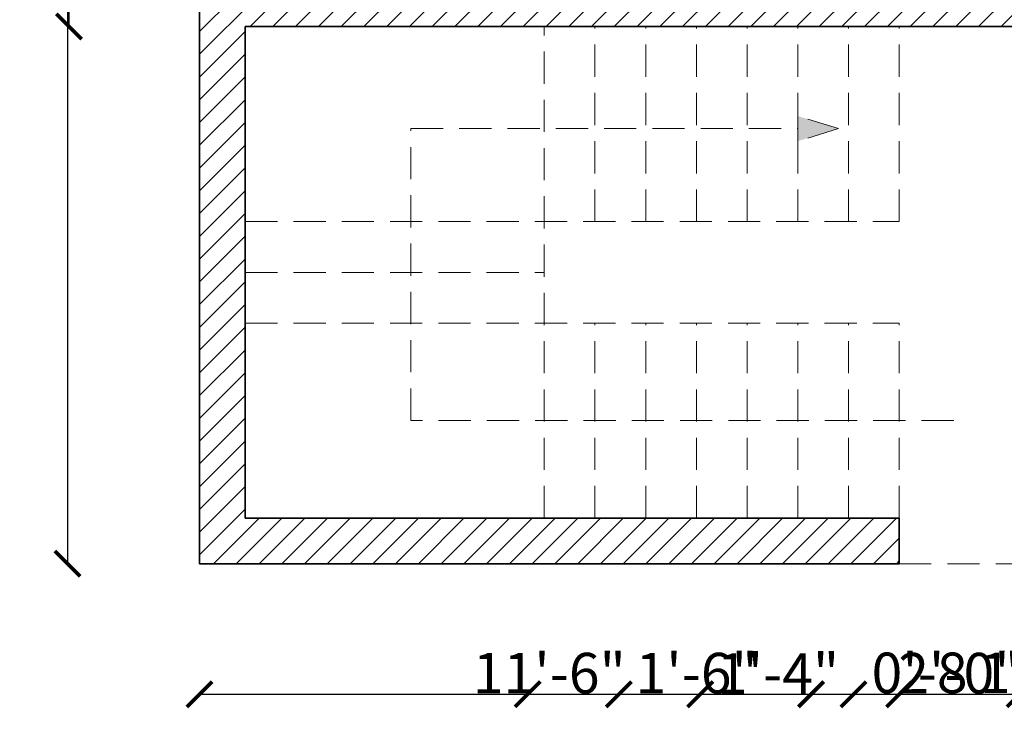
# Model space of a CAD drawing. Units: inches. Extents: x 2094 to 2639, y 1426 to 1997.
# Tile 1 of 8: x 2145 to 2339, y 1426 to 1567. Entities that reach past the tile are written whole.
import ezdxf

# ---------------------------------------------------------------- set-up
doc = ezdxf.new("R2010")
doc.units = ezdxf.units.IN
doc.linetypes.add('HIDDEN', pattern=[9.525, 6.35, -3.175])
for name, color, linetype, lineweight in [('A-ANNO-DIMS', 2, 'Continuous', 18), ('A-FLOR-HIDN', 7, 'HIDDEN', 18), ('A-WALL-PATT', 8, 'Continuous', 13), ('Steps', 50, 'HIDDEN', 18), ('Walls', 7, 'Continuous', 35)]:
    doc.layers.add(name, color=color, linetype=linetype, lineweight=lineweight)
doc.styles.get("Standard").update_dxf_attribs({"font": 'arial.ttf'})
doc.dimstyles.get("Standard").update_dxf_attribs({"dimtxt": 8, "dimasz": 5, "dimexe": 0.18, "dimexo": 0.0625, "dimgap": 0.09, "dimtad": 1, "dimdec": 1, "dimzin": 0, "dimdsep": 46, "dimlunit": 4, "dimtxsty": 'Standard', "dimblk": 'ARCHTICK', "dimcen": 0.09, "dimse1": 1, "dimse2": 1, "dimadec": 0, "dimazin": 0, "dimtfac": 1, "dimtdec": 1, "dimtofl": 0, "dimtmove": 0, "dimatfit": 3, "dimfxl": 1, "dimtolj": 1, "dimtzin": 0, "dimarcsym": 0})

# ---------------------------------------------------------------- blocks, each defined once
blk = doc.blocks.new('_ArchTick')
at = {"color": 0, "linetype": 'ByBlock', "const_width": 0.15}
blk.add_lwpolyline([(-0.5, -0.5), (0.5, 0.5)], dxfattribs=at)
blk = doc.blocks.new('*D14')
at = {"layer": 'A-ANNO-DIMS', "color": 0, "lineweight": -2, "transparency": 16777216}
blk.add_line((2154, 1928.9), (2154, 1459.9), dxfattribs=at)
at = {"layer": 'Defpoints', "color": 0, "transparency": 16777216}
for p in [(2180.06, 1928.9), (2154, 1459.9), (2180.06, 1459.9)]:
    blk.add_point(p, dxfattribs=at)
at = {"layer": 'A-ANNO-DIMS', "color": 0, "lineweight": -2, "transparency": 16777216, "xscale": 5, "yscale": 5, "zscale": 5}
for p, rotation in [((2154, 1928.9), 90), ((2154, 1459.9), 270)]:
    blk.add_blockref('_ArchTick', p, dxfattribs=dict(at, rotation=rotation))
at = {"layer": 'A-ANNO-DIMS', "color": 0, "transparency": 16777216, "insert": (2149.82, 1694.4), "char_height": 8, "attachment_point": 5, "rotation": 90}
blk.add_mtext('\\A1;39\'-1"', dxfattribs=at)
blk = doc.blocks.new('*D56')
at = {"layer": 'A-ANNO-DIMS', "color": 0, "lineweight": -2, "transparency": 16777216}
blk.add_line((2154.31, 1565.9), (2154.31, 1598.9), dxfattribs=at)
at = {"layer": 'Defpoints', "color": 0, "transparency": 16777216}
for p in [(2154.31, 1598.9), (2180.06, 1598.9), (2189.06, 1565.9)]:
    blk.add_point(p, dxfattribs=at)
at = {"layer": 'A-ANNO-DIMS', "color": 0, "lineweight": -2, "transparency": 16777216, "xscale": 5, "yscale": 5, "zscale": 5}
for p, rotation in [((2154.31, 1598.9), 90), ((2154.31, 1565.9), 270)]:
    blk.add_blockref('_ArchTick', p, dxfattribs=dict(at, rotation=rotation))
at = {"layer": 'A-ANNO-DIMS', "color": 0, "transparency": 16777216, "insert": (2150.13, 1582.4), "char_height": 8, "attachment_point": 5, "rotation": 90}
blk.add_mtext('\\A1;2\'-9"', dxfattribs=at)
blk = doc.blocks.new('*D61')
at = {"layer": 'A-ANNO-DIMS', "color": 0, "lineweight": -2, "transparency": 16777216}
blk.add_line((2318.06, 1434.15), (2341.83, 1434.15), dxfattribs=at)
at = {"layer": 'Defpoints', "color": 0, "transparency": 16777216}
for p in [(2318.06, 1565.9), (2341.83, 1565.9), (2341.83, 1434.15)]:
    blk.add_point(p, dxfattribs=at)
at = {"layer": 'A-ANNO-DIMS', "color": 0, "lineweight": -2, "transparency": 16777216, "xscale": 5, "yscale": 5, "zscale": 5, "rotation": 180}
blk.add_blockref('_ArchTick', (2318.06, 1434.15), dxfattribs=at)
at = {"layer": 'A-ANNO-DIMS', "color": 0, "lineweight": -2, "transparency": 16777216, "xscale": 5, "yscale": 5, "zscale": 5}
blk.add_blockref('_ArchTick', (2341.83, 1434.15), dxfattribs=at)
at = {"layer": 'A-ANNO-DIMS', "color": 0, "transparency": 16777216, "insert": (2329.94, 1438.32), "char_height": 8, "attachment_point": 5}
blk.add_mtext('\\A1;2\'-0"', dxfattribs=at)
blk = doc.blocks.new('*D71')
at = {"layer": 'A-ANNO-DIMS', "color": 0, "lineweight": -2, "transparency": 16777216}
for p, q in [((2300.69, 1434.15), (2309.06, 1434.15)), ((2309.06, 1434.15), (2354.14, 1434.15))]:
    blk.add_line(p, q, dxfattribs=at)
at = {"layer": 'Defpoints', "color": 0, "transparency": 16777216}
for p in [(2300.69, 1576.98), (2309.06, 1574.9), (2309.06, 1434.15)]:
    blk.add_point(p, dxfattribs=at)
at = {"layer": 'A-ANNO-DIMS', "color": 0, "lineweight": -2, "transparency": 16777216, "xscale": 5, "yscale": 5, "zscale": 5, "rotation": 180}
blk.add_blockref('_ArchTick', (2300.69, 1434.15), dxfattribs=at)
at = {"layer": 'A-ANNO-DIMS', "color": 0, "lineweight": -2, "transparency": 16777216, "xscale": 5, "yscale": 5, "zscale": 5}
blk.add_blockref('_ArchTick', (2309.06, 1434.15), dxfattribs=at)
at = {"layer": 'A-ANNO-DIMS', "color": 0, "transparency": 16777216, "insert": (2334.1, 1438.37), "char_height": 8, "attachment_point": 5}
blk.add_mtext('\\A1;0\'-8 1/2"', dxfattribs=at)
blk = doc.blocks.new('*D72')
at = {"layer": 'A-ANNO-DIMS', "color": 0, "lineweight": -2, "transparency": 16777216}
for p, q in [((2244.77, 1434.15), (2262.77, 1434.15)), ((2262.77, 1434.15), (2288.46, 1434.15))]:
    blk.add_line(p, q, dxfattribs=at)
at = {"layer": 'Defpoints', "color": 0, "transparency": 16777216}
for p in [(2244.77, 1576.36), (2262.77, 1576.36), (2262.77, 1434.15)]:
    blk.add_point(p, dxfattribs=at)
at = {"layer": 'A-ANNO-DIMS', "color": 0, "lineweight": -2, "transparency": 16777216, "xscale": 5, "yscale": 5, "zscale": 5, "rotation": 180}
blk.add_blockref('_ArchTick', (2244.77, 1434.15), dxfattribs=at)
at = {"layer": 'A-ANNO-DIMS', "color": 0, "lineweight": -2, "transparency": 16777216, "xscale": 5, "yscale": 5, "zscale": 5}
blk.add_blockref('_ArchTick', (2262.77, 1434.15), dxfattribs=at)
at = {"layer": 'A-ANNO-DIMS', "color": 0, "transparency": 16777216, "insert": (2278.12, 1438.32), "char_height": 8, "attachment_point": 5}
blk.add_mtext('\\A1;1\'-6"', dxfattribs=at)
blk = doc.blocks.new('*D73')
at = {"layer": 'A-ANNO-DIMS', "color": 0, "lineweight": -2, "transparency": 16777216}
for p, q in [((2262.77, 1434.15), (2278.83, 1434.15)), ((2278.83, 1434.15), (2304.53, 1434.15))]:
    blk.add_line(p, q, dxfattribs=at)
at = {"layer": 'Defpoints', "color": 0, "transparency": 16777216}
for p in [(2262.77, 1576.36), (2278.83, 1576.98), (2278.83, 1434.15)]:
    blk.add_point(p, dxfattribs=at)
at = {"layer": 'A-ANNO-DIMS', "color": 0, "lineweight": -2, "transparency": 16777216, "xscale": 5, "yscale": 5, "zscale": 5, "rotation": 180}
blk.add_blockref('_ArchTick', (2262.77, 1434.15), dxfattribs=at)
at = {"layer": 'A-ANNO-DIMS', "color": 0, "lineweight": -2, "transparency": 16777216, "xscale": 5, "yscale": 5, "zscale": 5}
blk.add_blockref('_ArchTick', (2278.83, 1434.15), dxfattribs=at)
at = {"layer": 'A-ANNO-DIMS', "color": 0, "transparency": 16777216, "insert": (2294.18, 1438.25), "char_height": 8, "attachment_point": 5}
blk.add_mtext('\\A1;1\'-4"', dxfattribs=at)
blk = doc.blocks.new('*D75')
at = {"layer": 'A-ANNO-DIMS', "color": 0, "lineweight": -2, "transparency": 16777216}
blk.add_line((2180.06, 1434.15), (2318.06, 1434.15), dxfattribs=at)
at = {"layer": 'Defpoints', "color": 0, "transparency": 16777216}
for p in [(2180.06, 1459.9), (2318.06, 1459.9), (2318.06, 1434.15)]:
    blk.add_point(p, dxfattribs=at)
at = {"layer": 'A-ANNO-DIMS', "color": 0, "lineweight": -2, "transparency": 16777216, "xscale": 5, "yscale": 5, "zscale": 5, "rotation": 180}
blk.add_blockref('_ArchTick', (2180.06, 1434.15), dxfattribs=at)
at = {"layer": 'A-ANNO-DIMS', "color": 0, "lineweight": -2, "transparency": 16777216, "xscale": 5, "yscale": 5, "zscale": 5}
blk.add_blockref('_ArchTick', (2318.06, 1434.15), dxfattribs=at)
at = {"layer": 'A-ANNO-DIMS', "color": 0, "transparency": 16777216, "insert": (2249.06, 1438.32), "char_height": 8, "attachment_point": 5}
blk.add_mtext('\\A1;11\'-6"', dxfattribs=at)
blk = doc.blocks.new('*D76')
at = {"layer": 'A-ANNO-DIMS', "color": 0, "lineweight": -2, "transparency": 16777216}
blk.add_line((2248.06, 1954.65), (2318.06, 1954.65), dxfattribs=at)
at = {"layer": 'Defpoints', "color": 0, "transparency": 16777216}
for p in [(2318.06, 1954.65), (2248.06, 1468.9), (2318.06, 1468.9)]:
    blk.add_point(p, dxfattribs=at)
at = {"layer": 'A-ANNO-DIMS', "color": 0, "lineweight": -2, "transparency": 16777216, "xscale": 5, "yscale": 5, "zscale": 5, "rotation": 180}
blk.add_blockref('_ArchTick', (2248.06, 1954.65), dxfattribs=at)
at = {"layer": 'A-ANNO-DIMS', "color": 0, "lineweight": -2, "transparency": 16777216, "xscale": 5, "yscale": 5, "zscale": 5}
blk.add_blockref('_ArchTick', (2318.06, 1954.65), dxfattribs=at)
at = {"layer": 'A-ANNO-DIMS', "color": 0, "transparency": 16777216, "insert": (2283.06, 1958.82), "char_height": 8, "attachment_point": 5}
blk.add_mtext('\\A1;5\'-10"', dxfattribs=at)
blk = doc.blocks.new('*D77')
at = {"layer": 'A-ANNO-DIMS', "color": 0, "lineweight": -2, "transparency": 16777216}
for p, q in [((2308.06, 1954.65), (2318.06, 1954.65)), ((2318.06, 1954.65), (2350.72, 1954.65))]:
    blk.add_line(p, q, dxfattribs=at)
at = {"layer": 'Defpoints', "color": 0, "transparency": 16777216}
for p in [(2318.06, 1954.65), (2308.06, 1468.9), (2318.06, 1468.9)]:
    blk.add_point(p, dxfattribs=at)
at = {"layer": 'A-ANNO-DIMS', "color": 0, "lineweight": -2, "transparency": 16777216, "xscale": 5, "yscale": 5, "zscale": 5, "rotation": 180}
blk.add_blockref('_ArchTick', (2308.06, 1954.65), dxfattribs=at)
at = {"layer": 'A-ANNO-DIMS', "color": 0, "lineweight": -2, "transparency": 16777216, "xscale": 5, "yscale": 5, "zscale": 5}
blk.add_blockref('_ArchTick', (2318.06, 1954.65), dxfattribs=at)
at = {"layer": 'A-ANNO-DIMS', "color": 0, "transparency": 16777216, "insert": (2336.89, 1958.82), "char_height": 8, "attachment_point": 5}
blk.add_mtext('\\A1;0\'-10"', dxfattribs=at)
blk = doc.blocks.new('*D78')
at = {"layer": 'A-ANNO-DIMS', "color": 0, "lineweight": -2, "transparency": 16777216}
for p, q in [((2562.81, 1507.4), (2562.81, 1552.48)), ((2562.81, 1468.9), (2562.81, 1507.4))]:
    blk.add_line(p, q, dxfattribs=at)
at = {"layer": 'Defpoints', "color": 0, "transparency": 16777216}
for p in [(2318.06, 1507.4), (2562.81, 1507.4), (2318.06, 1468.9)]:
    blk.add_point(p, dxfattribs=at)
at = {"layer": 'A-ANNO-DIMS', "color": 0, "lineweight": -2, "transparency": 16777216, "xscale": 5, "yscale": 5, "zscale": 5}
for p, rotation in [((2562.81, 1507.4), 90), ((2562.81, 1468.9), 270)]:
    blk.add_blockref('_ArchTick', p, dxfattribs=dict(at, rotation=rotation))
at = {"layer": 'A-ANNO-DIMS', "color": 0, "transparency": 16777216, "insert": (2558.58, 1532.44), "char_height": 8, "attachment_point": 5, "rotation": 90}
blk.add_mtext('\\A1;3\'-2 1/2"', dxfattribs=at)

msp = doc.modelspace()

# ---------------------------------------------------------------- hatches: boundary and pattern name
at = {"layer": 'A-WALL-PATT', "transparency": 33554585}
h = msp.add_hatch(dxfattribs=at)
h.set_pattern_fill('ANSI31', color=256)
h.paths.add_polyline_path([(2189.06, 1727.9), (2230.3, 1727.9, -0.022928), (2230.09, 1730.2), (2230.09, 1733.9), (2189.06, 1733.9), (2189.06, 1742.37), (2180.06, 1742.37), (2180.06, 1714.4), (2189.06, 1714.4)])
h.paths.add_polyline_path([(2456.51, 1574.9), (2413.83, 1574.9), (2413.83, 1565.9), (2456.51, 1565.9)])
h.paths.add_polyline_path([(2537.06, 1643.81), (2528.06, 1643.81), (2528.06, 1574.9), (2519.78, 1574.9), (2519.78, 1571.88), (2519.78, 1565.9), (2537.06, 1565.9)])
h.paths.add_polyline_path([(2339.06, 1928.9), (2300.94, 1928.9), (2300.94, 1919.9), (2309.06, 1919.9), (2309.06, 1776.3, -0.024186), (2312.62, 1776.64), (2318.06, 1776.64), (2318.06, 1778.9), (2336.06, 1778.9), (2336.06, 1787.9), (2318.06, 1787.9), (2318.06, 1835.9), (2384.06, 1835.9), (2384.06, 1787.9), (2366.06, 1787.9), (2366.06, 1778.9), (2479.64, 1778.9), (2479.64, 1784.88, -0.018603), (2479.89, 1787.9), (2390.06, 1787.9), (2390.06, 1847.57), (2385.61, 1847.57), (2384.06, 1847.57), (2384.06, 1841.9), (2318.06, 1841.9), (2318.06, 1919.9), (2339.06, 1919.9)])
h.paths.add_polyline_path([(2252.94, 1928.9), (2180.06, 1928.9), (2180.06, 1790.37), (2189.06, 1790.37), (2189.06, 1843.77), (2189.06, 1919.9), (2252.94, 1919.9)])
h.paths.add_polyline_path([(2472.33, 1928.9), (2363.06, 1928.9), (2363.06, 1919.9), (2384.06, 1919.9), (2384.06, 1876.38, -0.012802), (2385.61, 1876.49), (2390.06, 1876.49), (2390.06, 1919.9), (2472.33, 1919.9)], flags=17)
h.paths.add_polyline_path([(2537.06, 1928.9), (2520.33, 1928.9), (2520.33, 1919.9), (2528.06, 1919.9), (2528.06, 1905.95), (2528.06, 1787.9), (2518.5, 1787.9), (2518.5, 1784.88), (2518.5, 1778.9), (2528.06, 1778.9), (2528.06, 1715.81), (2537.06, 1715.81)])
h.paths.add_polyline_path([(2379.33, 1857.12), (2393.06, 1857.12), (2393.06, 1866.16), (2379.33, 1866.16)], flags=25)
h.paths.add_polyline_path([(2235.85, 1725.77), (2249.57, 1725.77), (2249.57, 1734.81), (2235.85, 1734.81)], flags=25)
h.paths.add_polyline_path([(2305.79, 1754.6), (2314.84, 1754.6), (2314.84, 1763.6), (2305.79, 1763.6)], flags=9)
h.paths.add_polyline_path([(2493.85, 1778.22), (2502.9, 1778.22), (2502.9, 1787.22), (2493.85, 1787.22)], flags=9)
h.paths.add_polyline_path([(2370.69, 1555.65), (2381.6, 1555.65), (2381.6, 1564.65), (2370.69, 1564.65)], flags=9)
h.paths.add_polyline_path([(2461.57, 1555.65), (2477.6, 1555.65), (2477.6, 1564.65), (2461.57, 1564.65)], flags=9)
h.paths.add_polyline_path([(2493.18, 1565.15), (2509.22, 1565.15), (2509.22, 1574.15), (2493.18, 1574.15)], flags=9)
h.paths.add_polyline_path([(2408.32, 1501.7), (2449.12, 1501.7), (2449.12, 1520.36), (2408.32, 1520.36)], flags=9)
h.paths.add_polyline_path([(2398.49, 1698.6), (2441.61, 1698.6), (2441.61, 1717.26), (2398.49, 1717.26)], flags=9)
h.paths.add_polyline_path([(2248.63, 1683.29), (2287.87, 1683.29), (2287.87, 1701.95), (2248.63, 1701.95)], flags=25)
h.paths.add_polyline_path([(2440.73, 1823.2), (2483.86, 1823.2), (2483.86, 1841.85), (2440.73, 1841.85)], flags=9)
h.paths.add_polyline_path([(2335.3, 1804.5), (2370.65, 1804.5), (2370.65, 1823.15), (2335.3, 1823.15)], flags=25)
h.paths.add_polyline_path([(2335.3, 1893.12), (2370.65, 1893.12), (2370.65, 1911.77), (2335.3, 1911.77)], flags=25)
h.paths.add_polyline_path([(2241.82, 1863.6), (2290.11, 1863.6), (2290.11, 1882.25), (2241.82, 1882.25)], flags=9)
h = msp.add_hatch(dxfattribs=at)
h.set_pattern_fill('ANSI31', color=256)
h.paths.add_polyline_path([(2318.06, 1741.32), (2312.62, 1741.32), (2309.06, 1741.32), (2309.06, 1733.9), (2254.12, 1733.9), (2254.12, 1730.2), (2254.12, 1727.9), (2309.06, 1727.9), (2309.06, 1676.9), (2189.06, 1676.9), (2189.06, 1690.4), (2180.06, 1690.4), (2180.06, 1646.9), (2189.06, 1646.9), (2189.06, 1670.9), (2309.06, 1670.9), (2309.06, 1640.9), (2318.06, 1640.9)])
h.paths.add_polyline_path([(2318.06, 1604.9), (2309.06, 1604.9), (2309.06, 1574.9), (2189.06, 1574.9), (2189.06, 1598.9), (2180.06, 1598.9), (2180.06, 1459.9), (2318.06, 1459.9), (2318.06, 1468.9), (2189.06, 1468.9), (2189.06, 1565.9), (2341.83, 1565.9), (2341.83, 1574.9), (2318.06, 1574.9)])
at = {"layer": 'Steps'}
h = msp.add_hatch(color=256, dxfattribs=at)
h.dxf.hatch_style = 1
h.paths.add_polyline_path([(2306.1, 1545.76), (2298.06, 1548.24), (2298.06, 1543.28)])

# ---------------------------------------------------------------- linework, layer by layer
at = {"layer": 'A-FLOR-HIDN'}
msp.add_line((2318.06, 1459.9), (2537.06, 1459.9), dxfattribs=at)
at = {"layer": 'Steps'}
for p, q in [((2248.06, 1468.9), (2248.06, 1565.9)), ((2258.06, 1527.4), (2258.06, 1565.9)), ((2268.06, 1527.4), (2268.06, 1565.9)), ((2278.06, 1527.4), (2278.06, 1565.9)), ((2288.06, 1527.4), (2288.06, 1565.9)), ((2298.06, 1527.4), (2298.06, 1565.9)), ((2308.06, 1527.4), (2308.06, 1565.9)), ((2318.06, 1527.4), (2318.06, 1565.9)), ((2298.06, 1548.24), (2298.06, 1543.28)), ((2306.1, 1545.76), (2298.06, 1548.24)), ((2221.76, 1488.15), (2221.76, 1545.76)), ((2221.76, 1545.76), (2298.06, 1545.76)), ((2306.1, 1545.76), (2298.06, 1543.28)), ((2189.06, 1527.4), (2318.06, 1527.4)), ((2189.06, 1517.4), (2248.06, 1517.4)), ((2189.06, 1507.4), (2318.06, 1507.4)), ((2258.06, 1468.9), (2258.06, 1507.4)), ((2268.06, 1468.9), (2268.06, 1507.4)), ((2278.06, 1468.9), (2278.06, 1507.4)), ((2288.06, 1468.9), (2288.06, 1507.4)), ((2298.06, 1468.9), (2298.06, 1507.4)), ((2308.06, 1468.9), (2308.06, 1507.4)), ((2318.06, 1468.9), (2318.06, 1507.4)), ((2328.82, 1488.15), (2221.76, 1488.15))]:
    msp.add_line(p, q, dxfattribs=at)
at = {"layer": 'Walls'}
for p, q in [((2180.06, 1928.9), (2180.06, 1459.9)), ((2189.06, 1565.9), (2480.92, 1565.9)), ((2189.06, 1565.9), (2189.06, 1468.9)), ((2189.06, 1468.9), (2318.06, 1468.9)), ((2318.06, 1468.9), (2318.06, 1459.9)), ((2180.06, 1459.9), (2318.06, 1459.9))]:
    msp.add_line(p, q, dxfattribs=at)

# ---------------------------------------------------------------- dimensions: what is measured, and where the dimension line sits
at = {"layer": 'A-ANNO-DIMS'}
for base, p1, p2, picture, middle in [((2318.06, 1954.65), (2248.06, 1468.9), (2318.06, 1468.9), '*D76', (2283.06, 1958.82)), ((2318.06, 1954.65), (2308.06, 1468.9), (2318.06, 1468.9), '*D77', (2336.89, 1958.82)), ((2262.77, 1434.15), (2244.77, 1576.36), (2262.77, 1576.36), '*D72', (2278.12, 1438.32)), ((2278.83, 1434.15), (2262.77, 1576.36), (2278.83, 1576.98), '*D73', (2294.18, 1438.25)), ((2309.06, 1434.15), (2300.69, 1576.98), (2309.06, 1574.9), '*D71', (2334.1, 1438.37)), ((2341.83, 1434.15), (2318.06, 1565.9), (2341.83, 1565.9), '*D61', (2329.94, 1438.32)), ((2318.06, 1434.15), (2180.06, 1459.9), (2318.06, 1459.9), '*D75', (2249.06, 1438.32))]:
    dim = msp.add_linear_dim(base=base, p1=p1, p2=p2, dimstyle='Standard', override={"dimdec": 1, "dimlfac": 1, "dimrnd": 0, "dimzin": 1, "dimdsep": 46, "dimlunit": 4, "dimfrac": 2}, dxfattribs=at)
    dim.commit()
    dim.dimension.update_dxf_attribs({"geometry": picture, "text_midpoint": middle})
for base, p1, p2, override, picture, middle in [((2154, 1459.9), (2180.06, 1928.9), (2180.06, 1459.9), {"dimclrd": 0, "dimclre": 0, "dimclrt": 0}, '*D14', (2149.82, 1694.4)), ((2154.31, 1598.9), (2189.06, 1565.9), (2180.06, 1598.9), {"dimdec": 1, "dimlfac": 1, "dimrnd": 0, "dimzin": 1, "dimdsep": 46, "dimlunit": 4, "dimfrac": 2}, '*D56', (2150.13, 1582.4)), ((2562.81, 1507.4), (2318.06, 1468.9), (2318.06, 1507.4), {"dimdec": 1, "dimlfac": 1, "dimrnd": 0, "dimzin": 1, "dimdsep": 46, "dimlunit": 4, "dimfrac": 2}, '*D78', (2558.58, 1532.44))]:
    dim = msp.add_linear_dim(base=base, p1=p1, p2=p2, angle=90, dimstyle='Standard', override=override, dxfattribs=at)
    dim.commit()
    dim.dimension.update_dxf_attribs({"geometry": picture, "text_midpoint": middle})

doc.saveas('drawing.dxf')
